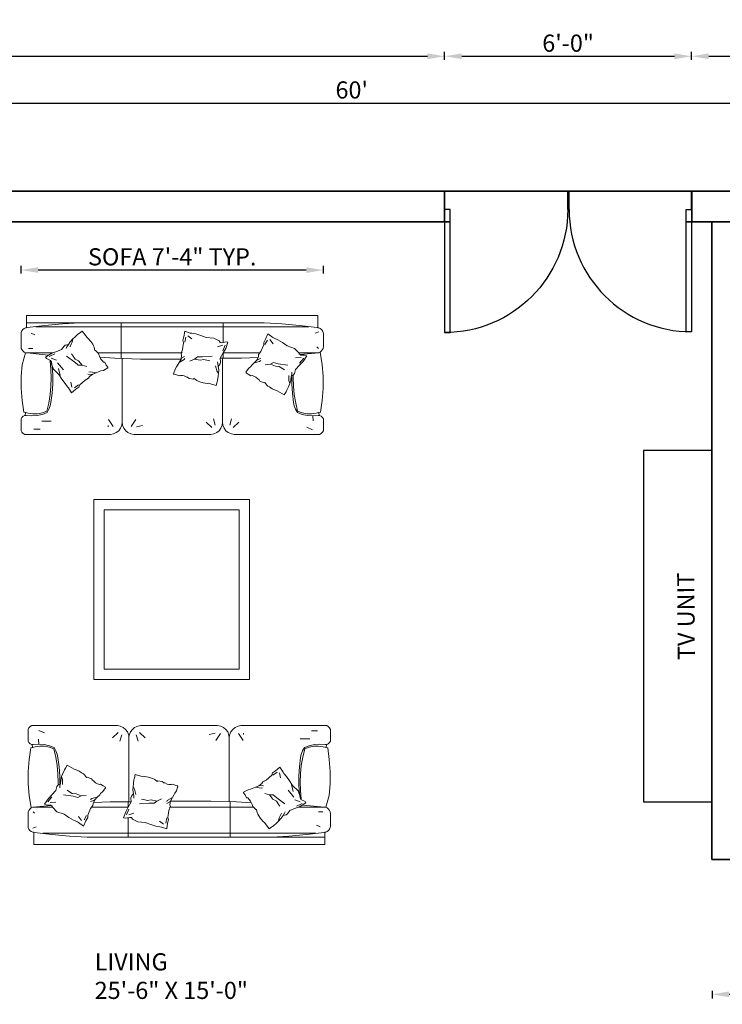
# Model space of a CAD drawing. Units: inches. Extents: x -48 to 817, y -530 to 78.
# Tile 6 of 7: x 266 to 470, y -225 to 62. Entities that reach past the tile are written whole.
import ezdxf

# ---------------------------------------------------------------- set-up
doc = ezdxf.new("R2010")
doc.units = ezdxf.units.IN
for name, color, linetype, lineweight in [('A-ANNO-DIMS', 2, 'Continuous', 18), ('A-AREA-IDEN', 7, 'Continuous', 18), ('A-DOOR', 3, 'Continuous', 25), ('A-FLOR-CASE', 8, 'Continuous', 25), ('A-WALL', 7, 'Continuous', 35), ('furn', 8, 'Continuous', 18), ('txt', 7, 'Continuous', 18)]:
    doc.layers.add(name, color=color, linetype=linetype, lineweight=lineweight)
doc.styles.get("Standard").update_dxf_attribs({"font": 'arial.ttf'})
doc.dimstyles.new('ISO-25', dxfattribs={"dimtxt": 5, "dimasz": 5, "dimexe": 1.25, "dimexo": 0.625, "dimtad": 1, "dimlunit": 3, "dimtxsty": 'Standard', "dimcen": 2.5, "dimadec": 0, "dimazin": 0, "dimtfac": 1, "dimtmove": 0, "dimatfit": 3, "dimfxl": 1, "dimfxlon": 1, "dimarcsym": 0})

# ---------------------------------------------------------------- blocks, each defined once
blk = doc.blocks.new('*U2')
for p, q in [((0, 0), (0, -6)), ((40, 0), (40, -6))]:
    blk.add_line(p, q)
blk.add_lwpolyline([(0, 0), (0, 40), (1.75, 40), (1.75, 0)], close=True)
blk.add_arc((0, 0), 40, 0, 90)
blk = doc.blocks.new('sofa-43')
at = {"color": 0, "linetype": 'ByBlock'}
for p, q in [((-0.015, 0.947), (-0.028, 0.939)), ((-0.028, 0.939), (-0.015, 0.947)), ((-0.003, 0.947), (-0.015, 0.947)), ((-0.015, 0.947), (-0.003, 0.947)), ((0.665, 0.947), (-0.003, 0.947)), ((-0.003, 0.947), (0.665, 0.947)), ((0.687, 0.942), (0.665, 0.947)), ((0.687, 0.942), (0.665, 0.947)), ((0.712, 0.932), (0.687, 0.942)), ((0.712, 0.932), (0.687, 0.942)), ((0.827, 0.942), (0.802, 0.932)), ((0.802, 0.932), (0.827, 0.942)), ((0.85, 0.947), (0.827, 0.942)), ((0.827, 0.942), (0.85, 0.947)), ((1.462, 0.947), (0.85, 0.947)), ((0.85, 0.947), (1.462, 0.947)), ((1.487, 0.942), (1.462, 0.947)), ((1.487, 0.942), (1.462, 0.947)), ((1.509, 0.932), (1.487, 0.942)), ((1.509, 0.932), (1.487, 0.942)), ((1.624, 0.942), (1.602, 0.932)), ((1.602, 0.932), (1.624, 0.942)), ((1.647, 0.947), (1.624, 0.942)), ((1.624, 0.942), (1.647, 0.947)), ((2.317, 0.947), (1.647, 0.947)), ((1.647, 0.947), (2.317, 0.947)), ((2.329, 0.947), (2.317, 0.947)), ((2.329, 0.947), (2.317, 0.947)), ((2.342, 0.939), (2.329, 0.947)), ((2.342, 0.939), (2.329, 0.947)), ((-0.038, 0.929), (-0.045, 0.917)), ((-0.045, 0.917), (-0.038, 0.929)), ((-0.045, 0.917), (-0.045, 0.824)), ((-0.045, 0.917), (-0.045, 0.824)), ((-0.028, 0.939), (-0.038, 0.929)), ((-0.038, 0.929), (-0.028, 0.939)), ((0.042, 0.909), (0.087, 0.889)), ((0.672, 0.892), (0.627, 0.849)), ((0.7, 0.874), (0.685, 0.824)), ((0.73, 0.917), (0.712, 0.932)), ((0.73, 0.917), (0.712, 0.932)), ((0.745, 0.897), (0.73, 0.917)), ((0.745, 0.897), (0.73, 0.917)), ((0.755, 0.872), (0.745, 0.897)), ((0.755, 0.872), (0.745, 0.897)), ((0.757, 0.849), (0.755, 0.872)), ((0.757, 0.849), (0.755, 0.872)), ((0.76, 0.872), (0.757, 0.849)), ((0.757, 0.849), (0.76, 0.872)), ((0.77, 0.897), (0.76, 0.872)), ((0.76, 0.872), (0.77, 0.897)), ((0.785, 0.917), (0.77, 0.897)), ((0.77, 0.897), (0.785, 0.917)), ((0.802, 0.932), (0.785, 0.917)), ((0.785, 0.917), (0.802, 0.932)), ((0.815, 0.874), (0.83, 0.824)), ((0.842, 0.892), (0.887, 0.849)), ((1.442, 0.887), (1.394, 0.877)), ((1.484, 0.884), (1.447, 0.829)), ((1.527, 0.917), (1.509, 0.932)), ((1.527, 0.917), (1.509, 0.932)), ((1.542, 0.897), (1.527, 0.917)), ((1.542, 0.897), (1.527, 0.917)), ((1.552, 0.872), (1.542, 0.897)), ((1.552, 0.872), (1.542, 0.897)), ((1.554, 0.849), (1.552, 0.872)), ((1.554, 0.849), (1.552, 0.872)), ((1.557, 0.872), (1.554, 0.849)), ((1.554, 0.849), (1.557, 0.872)), ((1.567, 0.897), (1.557, 0.872)), ((1.557, 0.872), (1.567, 0.897)), ((1.582, 0.917), (1.567, 0.897)), ((1.567, 0.897), (1.582, 0.917)), ((1.602, 0.932), (1.582, 0.917)), ((1.582, 0.917), (1.602, 0.932)), ((1.627, 0.884), (1.664, 0.829)), ((1.667, 0.887), (1.667, 0.877)), ((2.257, 0.904), (2.207, 0.904)), ((2.352, 0.929), (2.342, 0.939)), ((2.352, 0.929), (2.342, 0.939)), ((2.359, 0.917), (2.352, 0.929)), ((2.359, 0.917), (2.352, 0.929)), ((2.359, 0.824), (2.359, 0.917)), ((2.359, 0.917), (2.359, 0.824)), ((-0.045, 0.824), (-0.038, 0.812)), ((-0.045, 0.824), (-0.038, 0.812)), ((-0.038, 0.812), (-0.028, 0.802)), ((-0.038, 0.812), (-0.028, 0.802)), ((-0.028, 0.802), (-0.015, 0.797)), ((-0.028, 0.802), (-0.015, 0.797)), ((-0.015, 0.797), (-0.0064, 0.7737)), ((-0.015, 0.797), (-0.003, 0.797)), ((-0.0064, 0.7737), (-0.015, 0.797)), ((0.04, 0.799), (-0.003, 0.797)), ((0.04, 0.799), (0.037, 0.839)), ((0.082, 0.797), (0.04, 0.799)), ((0.125, 0.787), (0.082, 0.797)), ((0.162, 0.772), (0.125, 0.787)), ((0.757, 0.345), (0.757, 0.849)), ((1.554, 0.345), (1.554, 0.849)), ((2.194, 0.842), (2.119, 0.842)), ((2.152, 0.772), (2.189, 0.787)), ((2.189, 0.787), (2.232, 0.797)), ((2.232, 0.797), (2.274, 0.799)), ((2.274, 0.799), (2.317, 0.797)), ((2.329, 0.797), (2.317, 0.797)), ((2.3218, 0.7734), (2.329, 0.797)), ((2.3218, 0.7734), (2.329, 0.797)), ((2.329, 0.797), (2.342, 0.802)), ((2.342, 0.802), (2.329, 0.797)), ((2.342, 0.802), (2.352, 0.812)), ((2.352, 0.812), (2.342, 0.802)), ((2.352, 0.812), (2.359, 0.824)), ((2.359, 0.824), (2.352, 0.812)), ((-0.023, 0.769), (-0.035, 0.677)), ((-0.023, 0.769), (-0.035, 0.677)), ((0.012, 0.779), (-0.023, 0.769)), ((-0.0064, 0.7737), (-0.023, 0.769)), ((0.05, 0.782), (0.012, 0.779)), ((0.087, 0.782), (0.05, 0.782)), ((0.125, 0.774), (0.087, 0.782)), ((0.16, 0.762), (0.125, 0.774)), ((0.175, 0.697), (0.16, 0.762)), ((0.177, 0.747), (0.162, 0.772)), ((0.187, 0.719), (0.177, 0.747)), ((0.192, 0.692), (0.187, 0.719)), ((2.122, 0.692), (2.127, 0.719)), ((2.127, 0.719), (2.137, 0.747)), ((2.137, 0.747), (2.152, 0.772)), ((2.139, 0.697), (2.154, 0.762)), ((2.154, 0.762), (2.189, 0.774)), ((2.189, 0.774), (2.227, 0.782)), ((2.227, 0.782), (2.264, 0.782)), ((2.264, 0.782), (2.302, 0.779)), ((2.302, 0.779), (2.337, 0.769)), ((2.337, 0.769), (2.3218, 0.7734)), ((2.349, 0.677), (2.337, 0.769)), ((2.337, 0.769), (2.349, 0.677)), ((-0.035, 0.677), (-0.043, 0.582)), ((-0.035, 0.677), (-0.043, 0.582)), ((0.187, 0.629), (0.175, 0.697)), ((0.192, 0.562), (0.187, 0.629)), ((0.202, 0.619), (0.192, 0.692)), ((0.267, 0.632), (0.252, 0.607)), ((0.322, 0.599), (0.267, 0.632)), ((2.112, 0.619), (2.122, 0.692)), ((2.122, 0.562), (2.127, 0.629)), ((2.127, 0.629), (2.139, 0.697)), ((2.357, 0.582), (2.349, 0.677)), ((2.349, 0.677), (2.357, 0.582)), ((-0.043, 0.582), (-0.043, 0.484)), ((-0.043, 0.582), (-0.043, 0.484)), ((0.195, 0.497), (0.192, 0.562)), ((0.207, 0.547), (0.202, 0.619)), ((0.232, 0.567), (0.222, 0.542)), ((0.245, 0.594), (0.232, 0.567)), ((0.252, 0.607), (0.245, 0.594)), ((0.332, 0.597), (0.322, 0.599)), ((0.362, 0.584), (0.332, 0.597)), ((0.385, 0.569), (0.362, 0.584)), ((0.397, 0.562), (0.385, 0.569)), ((0.405, 0.554), (0.397, 0.562)), ((0.42, 0.534), (0.405, 0.554)), ((0.807, 0.557), (0.8, 0.529)), ((0.87, 0.539), (0.807, 0.557)), ((1.892, 0.552), (1.849, 0.514)), ((1.899, 0.572), (1.892, 0.552)), ((1.922, 0.587), (1.899, 0.572)), ((1.934, 0.577), (1.902, 0.552)), ((1.957, 0.617), (1.922, 0.587)), ((1.954, 0.572), (1.962, 0.532)), ((1.982, 0.577), (1.957, 0.617)), ((1.989, 0.567), (1.982, 0.577)), ((2.009, 0.542), (1.989, 0.567)), ((2.107, 0.547), (2.112, 0.619)), ((2.119, 0.497), (2.122, 0.562)), ((2.357, 0.484), (2.357, 0.582)), ((2.357, 0.582), (2.357, 0.484)), ((-0.043, 0.484), (-0.035, 0.392)), ((-0.043, 0.484), (-0.035, 0.392)), ((0.192, 0.472), (0.185, 0.462)), ((0.212, 0.487), (0.192, 0.472)), ((0.195, 0.482), (0.195, 0.497)), ((0.207, 0.492), (0.207, 0.547)), ((0.207, 0.467), (0.212, 0.487)), ((0.215, 0.514), (0.212, 0.487)), ((0.222, 0.542), (0.215, 0.514)), ((0.222, 0.542), (0.23, 0.519)), ((0.23, 0.519), (0.23, 0.497)), ((0.23, 0.497), (0.23, 0.477)), ((0.425, 0.537), (0.42, 0.534)), ((0.46, 0.524), (0.425, 0.537)), ((0.467, 0.512), (0.46, 0.524)), ((0.475, 0.507), (0.467, 0.512)), ((0.492, 0.492), (0.475, 0.507)), ((0.507, 0.484), (0.492, 0.492)), ((0.522, 0.479), (0.507, 0.484)), ((0.532, 0.482), (0.522, 0.479)), ((0.552, 0.467), (0.532, 0.482)), ((0.792, 0.484), (0.79, 0.462)), ((0.797, 0.517), (0.792, 0.484)), ((0.8, 0.529), (0.797, 0.517)), ((0.88, 0.542), (0.87, 0.539)), ((0.912, 0.537), (0.88, 0.542)), ((0.937, 0.529), (0.912, 0.537)), ((0.952, 0.524), (0.937, 0.529)), ((0.962, 0.519), (0.952, 0.524)), ((0.982, 0.502), (0.962, 0.519)), ((0.987, 0.507), (0.982, 0.502)), ((1.022, 0.502), (0.987, 0.507)), ((1.035, 0.492), (1.022, 0.502)), ((1.042, 0.492), (1.035, 0.492)), ((1.062, 0.482), (1.042, 0.492)), ((1.074, 0.477), (1.062, 0.482)), ((1.092, 0.477), (1.074, 0.477)), ((1.102, 0.482), (1.092, 0.477)), ((1.124, 0.472), (1.102, 0.482)), ((1.144, 0.467), (1.124, 0.472)), ((1.814, 0.487), (1.789, 0.467)), ((1.789, 0.467), (1.802, 0.47)), ((1.802, 0.47), (1.827, 0.467)), ((1.822, 0.499), (1.814, 0.487)), ((1.849, 0.514), (1.822, 0.499)), ((1.827, 0.504), (1.832, 0.502)), ((2.034, 0.507), (2.009, 0.542)), ((2.057, 0.47), (2.034, 0.507)), ((2.062, 0.422), (2.049, 0.479)), ((2.102, 0.427), (2.057, 0.47)), ((2.107, 0.474), (2.107, 0.547)), ((2.112, 0.405), (2.107, 0.474)), ((2.122, 0.43), (2.119, 0.497)), ((2.349, 0.392), (2.357, 0.484)), ((2.357, 0.484), (2.349, 0.392)), ((-0.035, 0.392), (-0.02, 0.292)), ((-0.035, 0.392), (-0.02, 0.292)), ((0.145, 0.395), (0.117, 0.367)), ((0.177, 0.43), (0.145, 0.395)), ((0.185, 0.462), (0.177, 0.43)), ((0.207, 0.452), (0.207, 0.467)), ((0.237, 0.397), (0.315, 0.385)), ((0.277, 0.425), (0.265, 0.432)), ((0.307, 0.407), (0.277, 0.425)), ((0.337, 0.405), (0.307, 0.407)), ((0.377, 0.387), (0.337, 0.405)), ((0.377, 0.387), (0.417, 0.392)), ((0.505, 0.377), (0.525, 0.397)), ((0.525, 0.397), (0.532, 0.407)), ((0.532, 0.407), (0.55, 0.422)), ((0.55, 0.422), (0.572, 0.452)), ((0.57, 0.457), (0.552, 0.467)), ((0.572, 0.452), (0.57, 0.457)), ((0.792, 0.407), (0.777, 0.385)), ((0.79, 0.462), (0.787, 0.432)), ((0.787, 0.432), (0.792, 0.407)), ((0.79, 0.462), (0.802, 0.442)), ((0.795, 0.382), (0.792, 0.407)), ((0.802, 0.442), (0.807, 0.42)), ((0.807, 0.42), (0.812, 0.4)), ((1.102, 0.375), (1.117, 0.4)), ((1.117, 0.4), (1.122, 0.41)), ((1.122, 0.41), (1.134, 0.427)), ((1.134, 0.427), (1.147, 0.465)), ((1.147, 0.465), (1.144, 0.467)), ((1.704, 0.437), (1.669, 0.417)), ((1.669, 0.417), (1.669, 0.412)), ((1.669, 0.412), (1.682, 0.395)), ((1.682, 0.395), (1.692, 0.372)), ((1.724, 0.442), (1.704, 0.437)), ((1.737, 0.447), (1.724, 0.442)), ((1.762, 0.457), (1.737, 0.447)), ((1.789, 0.467), (1.762, 0.457)), ((1.762, 0.457), (1.807, 0.45)), ((1.807, 0.45), (1.819, 0.452)), ((1.874, 0.397), (1.837, 0.407)), ((1.874, 0.397), (1.902, 0.362)), ((1.904, 0.397), (1.874, 0.397)), ((1.932, 0.372), (1.904, 0.397)), ((2.069, 0.377), (2.022, 0.432)), ((2.119, 0.382), (2.102, 0.427)), ((2.117, 0.375), (2.112, 0.405)), ((2.127, 0.362), (2.122, 0.43)), ((2.322, 0.297), (2.349, 0.392)), ((2.349, 0.392), (2.322, 0.297)), ((0.117, 0.367), (0.087, 0.322)), ((0.087, 0.322), (0.1, 0.317)), ((0.1, 0.317), (0.135, 0.315)), ((0.112, 0.34), (0.145, 0.38)), ((0.132, 0.335), (0.177, 0.337)), ((0.135, 0.315), (0.147, 0.307)), ((0.315, 0.385), (0.352, 0.375)), ((0.352, 0.375), (0.377, 0.387)), ((0.462, 0.367), (0.452, 0.36)), ((0.477, 0.35), (0.452, 0.342)), ((0.505, 0.377), (0.462, 0.367)), ((0.47, 0.312), (0.472, 0.327)), ((0.472, 0.327), (0.485, 0.357)), ((0.607, 0.34), (0.475, 0.335)), ((0.485, 0.357), (0.477, 0.35)), ((0.485, 0.357), (0.505, 0.377)), ((0.775, 0.34), (0.607, 0.34)), ((0.775, 0.34), (0.752, 0.297)), ((0.752, 0.297), (0.752, 0.34)), ((0.777, 0.385), (0.772, 0.372)), ((0.772, 0.372), (0.775, 0.34)), ((0.797, 0.37), (0.795, 0.382)), ((0.84, 0.325), (0.917, 0.33)), ((0.872, 0.36), (0.857, 0.362)), ((0.905, 0.35), (0.872, 0.36)), ((0.935, 0.357), (0.905, 0.35)), ((0.917, 0.33), (0.957, 0.33)), ((0.98, 0.347), (0.935, 0.357)), ((0.957, 0.33), (0.98, 0.347)), ((0.98, 0.347), (1.017, 0.365)), ((1.062, 0.352), (1.057, 0.342)), ((1.082, 0.34), (1.059, 0.327)), ((1.102, 0.375), (1.062, 0.352)), ((1.087, 0.347), (1.082, 0.34)), ((1.082, 0.317), (1.087, 0.347)), ((1.087, 0.302), (1.082, 0.317)), ((1.087, 0.347), (1.102, 0.375)), ((1.409, 0.347), (1.087, 0.347)), ((1.612, 0.34), (1.409, 0.347)), ((1.562, 0.06), (1.562, 0.34)), ((1.732, 0.332), (1.612, 0.34)), ((1.692, 0.372), (1.702, 0.372)), ((1.702, 0.372), (1.714, 0.36)), ((1.714, 0.36), (1.724, 0.347)), ((1.724, 0.347), (1.734, 0.325)), ((1.734, 0.325), (1.737, 0.32)), ((1.737, 0.32), (1.742, 0.302)), ((1.902, 0.362), (1.929, 0.347)), ((1.929, 0.347), (1.949, 0.317)), ((1.997, 0.325), (1.932, 0.372)), ((1.949, 0.317), (1.957, 0.307)), ((2.119, 0.34), (2.077, 0.357)), ((2.134, 0.327), (2.089, 0.305)), ((2.117, 0.317), (2.114, 0.317)), ((2.117, 0.37), (2.119, 0.382)), ((2.124, 0.36), (2.117, 0.37)), ((2.119, 0.302), (2.164, 0.332)), ((2.157, 0.342), (2.124, 0.36)), ((2.129, 0.357), (2.127, 0.362)), ((2.144, 0.315), (2.137, 0.317)), ((2.137, 0.315), (2.137, 0.317)), ((2.309, 0.297), (2.144, 0.315)), ((2.164, 0.332), (2.157, 0.342)), ((-0.043, 0.262), (-0.045, 0.247)), ((-0.043, 0.262), (-0.045, 0.247)), ((-0.045, 0.247), (-0.045, 0.147)), ((-0.045, 0.247), (-0.045, 0.147)), ((-0.038, 0.272), (-0.043, 0.262)), ((-0.038, 0.272), (-0.043, 0.262)), ((-0.03, 0.282), (-0.038, 0.272)), ((-0.03, 0.282), (-0.038, 0.272)), ((-0.02, 0.292), (-0.03, 0.282)), ((-0.02, 0.292), (-0.03, 0.282)), ((-0.008, 0.297), (-0.02, 0.292)), ((0.14, 0.312), (-0.008, 0.297)), ((-0.008, 0.297), (0.15, 0.297)), ((0.005, 0.297), (-0.008, 0.297)), ((-0.005, 0.262), (0.007, 0.25)), ((0.147, 0.307), (0.152, 0.295)), ((0.152, 0.295), (0.185, 0.262)), ((0.185, 0.262), (0.242, 0.242)), ((0.242, 0.242), (0.28, 0.215)), ((0.43, 0.235), (0.452, 0.287)), ((0.43, 0.215), (0.43, 0.235)), ((0.452, 0.287), (0.47, 0.312)), ((0.46, 0.297), (0.752, 0.297)), ((0.467, 0.307), (0.462, 0.307)), ((0.732, 0.262), (0.715, 0.212)), ((0.752, 0.297), (0.732, 0.262)), ((0.737, 0.237), (0.755, 0.282)), ((0.755, 0.237), (0.797, 0.25)), ((1.067, 0.217), (1.074, 0.272)), ((1.074, 0.272), (1.087, 0.302)), ((1.084, 0.297), (1.079, 0.292)), ((1.0855, 0.2985), (1.084, 0.297)), ((1.084, 0.297), (1.0848, 0.297)), ((1.084, 0.297), (1.562, 0.297)), ((1.0848, 0.297), (1.0855, 0.2985)), ((1.562, 0.297), (1.747, 0.297)), ((1.742, 0.302), (1.767, 0.28)), ((1.767, 0.28), (1.772, 0.28)), ((1.772, 0.28), (1.777, 0.252)), ((1.777, 0.252), (1.782, 0.242)), ((1.782, 0.242), (1.789, 0.23)), ((1.959, 0.23), (1.969, 0.25)), ((1.994, 0.25), (1.982, 0.232)), ((1.982, 0.232), (2.007, 0.237)), ((1.999, 0.262), (1.994, 0.25)), ((2.007, 0.237), (2.017, 0.245)), ((2.017, 0.245), (2.037, 0.272)), ((2.037, 0.272), (2.082, 0.29)), ((2.082, 0.29), (2.119, 0.302)), ((2.104, 0.297), (2.309, 0.297)), ((2.299, 0.262), (2.264, 0.262)), ((2.322, 0.297), (2.309, 0.297)), ((2.334, 0.292), (2.322, 0.297)), ((2.334, 0.292), (2.322, 0.297)), ((2.344, 0.282), (2.334, 0.292)), ((2.344, 0.282), (2.334, 0.292)), ((2.352, 0.272), (2.344, 0.282)), ((2.352, 0.272), (2.344, 0.282)), ((2.357, 0.262), (2.352, 0.272)), ((2.357, 0.262), (2.352, 0.272)), ((2.359, 0.247), (2.357, 0.262)), ((2.359, 0.247), (2.357, 0.262)), ((2.359, 0.147), (2.359, 0.247)), ((2.359, 0.147), (2.359, 0.247)), ((0.28, 0.215), (0.317, 0.195)), ((0.317, 0.195), (0.347, 0.182)), ((0.347, 0.182), (0.357, 0.175)), ((0.38, 0.192), (0.355, 0.225)), ((0.357, 0.175), (0.397, 0.147)), ((0.397, 0.147), (0.415, 0.19)), ((0.4, 0.197), (0.42, 0.232)), ((0.415, 0.19), (0.43, 0.215)), ((0.715, 0.212), (0.727, 0.21)), ((0.727, 0.21), (0.765, 0.217)), ((0.752, 0.06), (0.752, 0.215)), ((0.765, 0.217), (0.777, 0.215)), ((0.777, 0.215), (0.785, 0.202)), ((0.785, 0.202), (0.827, 0.18)), ((0.827, 0.18), (0.887, 0.175)), ((0.887, 0.175), (0.93, 0.16)), ((0.93, 0.16), (0.97, 0.147)), ((1.032, 0.162), (1, 0.187)), ((1.05, 0.172), (1.057, 0.212)), ((1.057, 0.125), (1.064, 0.17)), ((1.064, 0.17), (1.072, 0.197)), ((1.072, 0.197), (1.067, 0.217)), ((1.789, 0.23), (1.804, 0.207)), ((1.804, 0.207), (1.827, 0.182)), ((1.827, 0.182), (1.834, 0.177)), ((1.834, 0.177), (1.872, 0.125)), ((1.907, 0.15), (1.929, 0.17)), ((1.929, 0.17), (1.947, 0.187)), ((1.947, 0.187), (1.952, 0.212)), ((1.947, 0.187), (1.967, 0.21)), ((1.952, 0.212), (1.959, 0.23)), ((1.967, 0.21), (1.982, 0.232)), ((-0.045, 0.147), (-0.043, 0.135)), ((-0.045, 0.147), (-0.043, 0.135)), ((-0.043, 0.135), (-0.038, 0.122)), ((-0.043, 0.135), (-0.038, 0.122)), ((-0.038, 0.122), (-0.03, 0.112)), ((-0.038, 0.122), (-0.03, 0.112)), ((-0.03, 0.112), (-0.02, 0.105)), ((-0.03, 0.112), (-0.02, 0.105)), ((-0.02, 0.105), (-0.008, 0.1)), ((-0.02, 0.105), (-0.008, 0.1)), ((-0.008, 0.132), (0.02, 0.142)), ((-0.008, 0.1), (0, 0.0982)), ((-0.008, 0.1), (0.005, 0.097)), ((0, 0.1), (0, 0)), ((0, 0.0982), (0, 0)), ((0.005, 0.097), (0.145, 0.08)), ((0.072, 0.09), (0.752, 0.09)), ((0.145, 0.08), (0.285, 0.067)), ((0.752, 0.09), (1.562, 0.09)), ((0.97, 0.147), (1.002, 0.142)), ((1.002, 0.142), (1.015, 0.14)), ((1.015, 0.14), (1.057, 0.125)), ((1.562, 0.09), (2.242, 0.09)), ((1.872, 0.125), (1.894, 0.142)), ((1.894, 0.142), (1.907, 0.15)), ((2.029, 0.067), (2.169, 0.08)), ((2.169, 0.08), (2.309, 0.097)), ((2.277, 0.142), (2.249, 0.155)), ((2.309, 0.097), (2.322, 0.1)), ((2.314, 0.0982), (2.322, 0.1)), ((2.314, 0.1), (2.314, 0)), ((2.314, 0), (2.314, 0.0982)), ((2.322, 0.1), (2.334, 0.105)), ((2.322, 0.1), (2.334, 0.105)), ((2.334, 0.105), (2.344, 0.112)), ((2.334, 0.105), (2.344, 0.112)), ((2.344, 0.112), (2.352, 0.122)), ((2.344, 0.112), (2.352, 0.122)), ((2.352, 0.122), (2.357, 0.135)), ((2.352, 0.122), (2.357, 0.135)), ((2.357, 0.135), (2.359, 0.147)), ((2.357, 0.135), (2.359, 0.147)), ((0, 0), (2.314, 0)), ((0, 0), (2.314, 0)), ((0.285, 0.067), (0.425, 0.06)), ((0.425, 0.06), (2.314, 0.06)), ((1.889, 0.06), (2.029, 0.067))]:
    blk.add_line(p, q, dxfattribs=at)
blk = doc.blocks.new('*D9')
at = {"layer": 'A-ANNO-DIMS', "color": 0, "lineweight": -2, "transparency": 16777216}
for p, q in [((2.43, 36.38), (2.43, 38.63)), ((7.43, 37.38), (717.43, 37.38)), ((722.43, 36.38), (722.43, 38.63))]:
    blk.add_line(p, q, dxfattribs=at)
at = {"layer": 'A-ANNO-DIMS', "color": 0, "transparency": 16777216}
for points in [[(7.43, 38.21), (7.43, 36.54), (2.43, 37.38)], [(717.43, 38.21), (717.43, 36.54), (722.43, 37.38)]]:
    blk.add_solid(points, dxfattribs=at)
at = {"layer": 'Defpoints', "color": 0, "transparency": 16777216}
for p in [(722.43, 37.38), (2.43, 11.72), (722.43, 11.72)]:
    blk.add_point(p, dxfattribs=at)
at = {"layer": 'A-ANNO-DIMS', "color": 0, "transparency": 16777216, "insert": (362.43, 40.55), "char_height": 5, "attachment_point": 5}
blk.add_mtext("60'", dxfattribs=at)
blk = doc.blocks.new('*D26')
at = {"layer": 'A-ANNO-DIMS', "color": 0, "lineweight": -2, "transparency": 16777216}
for p, q in [((266.04, -12.33), (266.04, -10.08)), ((349.18, -11.33), (271.04, -11.33)), ((354.18, -12.33), (354.18, -10.08))]:
    blk.add_line(p, q, dxfattribs=at)
at = {"layer": 'A-ANNO-DIMS', "color": 0, "transparency": 16777216}
for points in [[(271.04, -10.5), (271.04, -12.17), (266.04, -11.33)], [(349.18, -10.5), (349.18, -12.17), (354.18, -11.33)]]:
    blk.add_solid(points, dxfattribs=at)
at = {"layer": 'Defpoints', "color": 0, "transparency": 16777216}
for p in [(266.04, -11.33), (266.04, -24.56), (354.18, -24.56)]:
    blk.add_point(p, dxfattribs=at)
at = {"layer": 'A-ANNO-DIMS', "color": 0, "transparency": 16777216, "insert": (310.11, -8.12), "char_height": 5, "attachment_point": 5}
blk.add_mtext('SOFA 7\'-4" TYP.', dxfattribs=at)
blk = doc.blocks.new('*D27')
at = {"layer": 'A-ANNO-DIMS', "color": 0, "lineweight": -2, "transparency": 16777216}
for p, q in [((253.82, -24.56), (251.57, -24.56)), ((252.82, -29.56), (252.82, -54.28)), ((253.82, -59.28), (251.57, -59.28)), ((252.82, -59.28), (252.82, -111.62))]:
    blk.add_line(p, q, dxfattribs=at)
at = {"layer": 'A-ANNO-DIMS', "color": 0, "transparency": 16777216}
for points in [[(251.99, -29.56), (253.65, -29.56), (252.82, -24.56)], [(251.99, -54.28), (253.65, -54.28), (252.82, -59.28)]]:
    blk.add_solid(points, dxfattribs=at)
at = {"layer": 'Defpoints', "color": 0, "transparency": 16777216}
for p in [(266.04, -24.56), (252.82, -59.28), (266.04, -59.28)]:
    blk.add_point(p, dxfattribs=at)
at = {"layer": 'A-ANNO-DIMS', "color": 0, "transparency": 16777216, "insert": (249.61, -87.95), "char_height": 5, "attachment_point": 5, "rotation": 90}
blk.add_mtext('2\'-10 1/2" TYP.', dxfattribs=at)
blk = doc.blocks.new('*D44')
at = {"layer": 'A-ANNO-DIMS', "color": 0, "lineweight": -2, "transparency": 16777216}
for p, q in [((389.5, 50.02), (389.5, 52.27)), ((461.47, 50.02), (461.47, 52.27)), ((394.5, 51.02), (456.47, 51.02))]:
    blk.add_line(p, q, dxfattribs=at)
at = {"layer": 'A-ANNO-DIMS', "color": 0, "transparency": 16777216}
for points in [[(394.5, 51.86), (394.5, 50.19), (389.5, 51.02)], [(456.47, 51.86), (456.47, 50.19), (461.47, 51.02)]]:
    blk.add_solid(points, dxfattribs=at)
at = {"layer": 'Defpoints', "color": 0, "transparency": 16777216}
for p in [(461.47, 51.02), (389.5, 11.72), (461.47, 11.72)]:
    blk.add_point(p, dxfattribs=at)
at = {"layer": 'A-ANNO-DIMS', "color": 0, "transparency": 16777216, "insert": (425.49, 54.2), "char_height": 5, "attachment_point": 5}
blk.add_mtext('6\'-0"', dxfattribs=at)
blk = doc.blocks.new('*D48')
at = {"layer": 'A-ANNO-DIMS', "color": 0, "lineweight": -2, "transparency": 16777216}
for p, q in [((105.2, 50.02), (105.2, 52.27)), ((389.5, 50.02), (389.5, 52.27)), ((110.2, 51.02), (384.5, 51.02))]:
    blk.add_line(p, q, dxfattribs=at)
at = {"layer": 'A-ANNO-DIMS', "color": 0, "transparency": 16777216}
for points in [[(110.2, 51.86), (110.2, 50.19), (105.2, 51.02)], [(384.5, 51.86), (384.5, 50.19), (389.5, 51.02)]]:
    blk.add_solid(points, dxfattribs=at)
at = {"layer": 'Defpoints', "color": 0, "transparency": 16777216}
for p in [(389.5, 51.02), (105.2, 11.72), (389.5, 11.72)]:
    blk.add_point(p, dxfattribs=at)
at = {"layer": 'A-ANNO-DIMS', "color": 0, "transparency": 16777216, "insert": (247.35, 54.24), "char_height": 5, "attachment_point": 5}
blk.add_mtext('23\'-8 1/2"', dxfattribs=at)
blk = doc.blocks.new('*D49')
at = {"layer": 'A-ANNO-DIMS', "color": 0, "lineweight": -2, "transparency": 16777216}
for p, q in [((461.47, 50.02), (461.47, 52.27)), ((509.58, 50.02), (509.58, 52.27)), ((466.47, 51.02), (504.58, 51.02))]:
    blk.add_line(p, q, dxfattribs=at)
at = {"layer": 'A-ANNO-DIMS', "color": 0, "transparency": 16777216}
for points in [[(466.47, 51.86), (466.47, 50.19), (461.47, 51.02)], [(504.58, 51.86), (504.58, 50.19), (509.58, 51.02)]]:
    blk.add_solid(points, dxfattribs=at)
at = {"layer": 'Defpoints', "color": 0, "transparency": 16777216}
for p in [(509.58, 51.02), (461.47, 11.72), (509.58, 11.72)]:
    blk.add_point(p, dxfattribs=at)
at = {"layer": 'A-ANNO-DIMS', "color": 0, "transparency": 16777216, "insert": (485.53, 54.2), "char_height": 5, "attachment_point": 5}
blk.add_mtext('4\'-0"', dxfattribs=at)
blk = doc.blocks.new('*D58')
at = {"layer": 'A-ANNO-DIMS', "color": 0, "lineweight": -2, "transparency": 16777216}
for p, q in [((811.62, -33.28), (813.87, -33.28)), ((812.62, -38.28), (812.62, -100.61)), ((811.62, -105.61), (813.87, -105.61))]:
    blk.add_line(p, q, dxfattribs=at)
at = {"layer": 'A-ANNO-DIMS', "color": 0, "transparency": 16777216}
for points in [[(811.79, -38.28), (813.45, -38.28), (812.62, -33.28)], [(811.79, -100.61), (813.45, -100.61), (812.62, -105.61)]]:
    blk.add_solid(points, dxfattribs=at)
at = {"layer": 'Defpoints', "color": 0, "transparency": 16777216}
for p in [(161.43, -33.28), (161.43, -105.61), (812.62, -105.61)]:
    blk.add_point(p, dxfattribs=at)
at = {"layer": 'A-ANNO-DIMS', "color": 0, "transparency": 16777216, "insert": (809.41, -69.44), "char_height": 5, "attachment_point": 5, "rotation": 90}
blk.add_mtext('6\'-0 1/2"', dxfattribs=at)
blk = doc.blocks.new('*D60')
at = {"layer": 'A-ANNO-DIMS', "color": 0, "lineweight": -2, "transparency": 16777216}
for p, q in [((467.43, -221.58), (467.43, -223.83)), ((511.25, -222.58), (472.43, -222.58)), ((516.25, -221.58), (516.25, -223.83))]:
    blk.add_line(p, q, dxfattribs=at)
at = {"layer": 'A-ANNO-DIMS', "color": 0, "transparency": 16777216}
for points in [[(472.43, -221.74), (472.43, -223.41), (467.43, -222.58)], [(511.25, -221.74), (511.25, -223.41), (516.25, -222.58)]]:
    blk.add_solid(points, dxfattribs=at)
at = {"layer": 'Defpoints', "color": 0, "transparency": 16777216}
for p in [(467.43, -183.28), (516.25, -183.28), (467.43, -222.58)]:
    blk.add_point(p, dxfattribs=at)
at = {"layer": 'A-ANNO-DIMS', "color": 0, "transparency": 16777216, "insert": (491.84, -219.44), "char_height": 5, "attachment_point": 5}
blk.add_mtext('4\'-1"', dxfattribs=at)
blk = doc.blocks.new('*D68')
at = {"layer": 'A-ANNO-DIMS', "color": 0, "lineweight": -2, "transparency": 16777216}
for p, q in [((-35.87, -153.28), (-38.12, -153.28)), ((-36.87, -158.28), (-36.87, -172.28)), ((-35.87, -177.28), (-38.12, -177.28))]:
    blk.add_line(p, q, dxfattribs=at)
at = {"layer": 'A-ANNO-DIMS', "color": 0, "transparency": 16777216}
for points in [[(-37.71, -158.28), (-36.04, -158.28), (-36.87, -153.28)], [(-37.71, -172.28), (-36.04, -172.28), (-36.87, -177.28)]]:
    blk.add_solid(points, dxfattribs=at)
at = {"layer": 'Defpoints', "color": 0, "transparency": 16777216}
for p in [(570.33, -153.28), (-36.87, -177.28), (570.33, -177.28)]:
    blk.add_point(p, dxfattribs=at)
at = {"layer": 'A-ANNO-DIMS', "color": 0, "transparency": 16777216, "insert": (-40.05, -165.28), "char_height": 5, "attachment_point": 5, "rotation": 90}
blk.add_mtext('2\'-0"', dxfattribs=at)
blk = doc.blocks.new('*D74')
at = {"layer": 'A-ANNO-DIMS', "color": 0, "lineweight": -2, "transparency": 16777216}
for p, q in [((811.62, -47.3), (813.87, -47.3)), ((812.62, -52.3), (812.62, -94.77)), ((811.62, -99.77), (813.87, -99.77))]:
    blk.add_line(p, q, dxfattribs=at)
at = {"layer": 'A-ANNO-DIMS', "color": 0, "transparency": 16777216}
for points in [[(811.79, -52.3), (813.45, -52.3), (812.62, -47.3)], [(811.79, -94.77), (813.45, -94.77), (812.62, -99.77)]]:
    blk.add_solid(points, dxfattribs=at)
at = {"layer": 'Defpoints', "color": 0, "transparency": 16777216}
for p in [(44.85, -47.3), (44.85, -99.77), (812.62, -99.77)]:
    blk.add_point(p, dxfattribs=at)
at = {"layer": 'A-ANNO-DIMS', "color": 0, "transparency": 16777216, "insert": (809.41, -73.53), "char_height": 5, "attachment_point": 5, "rotation": 90}
blk.add_mtext('4\'-4 1/2"', dxfattribs=at)
blk = doc.blocks.new('*D75')
at = {"layer": 'A-ANNO-DIMS', "color": 0, "lineweight": -2, "transparency": 16777216}
for p, q in [((287.29, -506.59), (287.29, -508.84)), ((292.29, -507.59), (327.6, -507.59)), ((332.6, -506.59), (332.6, -508.84))]:
    blk.add_line(p, q, dxfattribs=at)
at = {"layer": 'A-ANNO-DIMS', "color": 0, "transparency": 16777216}
for points in [[(292.29, -506.76), (292.29, -508.42), (287.29, -507.59)], [(327.6, -506.76), (327.6, -508.42), (332.6, -507.59)]]:
    blk.add_solid(points, dxfattribs=at)
at = {"layer": 'Defpoints', "color": 0, "transparency": 16777216}
for p in [(287.29, -130.76), (332.6, -130.76), (332.6, -507.59)]:
    blk.add_point(p, dxfattribs=at)
at = {"layer": 'A-ANNO-DIMS', "color": 0, "transparency": 16777216, "insert": (309.94, -504.38), "char_height": 5, "attachment_point": 5}
blk.add_mtext('3\'-9 1/2"', dxfattribs=at)
blk = doc.blocks.new('*D76')
at = {"layer": 'A-ANNO-DIMS', "color": 0, "lineweight": -2, "transparency": 16777216}
for p, q in [((811.62, -78.22), (813.87, -78.22)), ((812.62, -83.22), (812.62, -125.76)), ((811.62, -130.76), (813.87, -130.76))]:
    blk.add_line(p, q, dxfattribs=at)
at = {"layer": 'A-ANNO-DIMS', "color": 0, "transparency": 16777216}
for points in [[(811.79, -83.22), (813.45, -83.22), (812.62, -78.22)], [(811.79, -125.76), (813.45, -125.76), (812.62, -130.76)]]:
    blk.add_solid(points, dxfattribs=at)
at = {"layer": 'Defpoints', "color": 0, "transparency": 16777216}
for p in [(332.6, -78.22), (332.6, -130.76), (812.62, -130.76)]:
    blk.add_point(p, dxfattribs=at)
at = {"layer": 'A-ANNO-DIMS', "color": 0, "transparency": 16777216, "insert": (809.41, -104.49), "char_height": 5, "attachment_point": 5, "rotation": 90}
blk.add_mtext('4\'-4 1/2"', dxfattribs=at)
blk = doc.blocks.new('*D79')
at = {"layer": 'A-ANNO-DIMS', "color": 0, "lineweight": -2, "transparency": 16777216}
for p, q in [((447.47, -506.59), (447.47, -508.84)), ((452.47, -507.59), (462.43, -507.59)), ((467.43, -506.59), (467.43, -508.84))]:
    blk.add_line(p, q, dxfattribs=at)
at = {"layer": 'A-ANNO-DIMS', "color": 0, "transparency": 16777216}
for points in [[(452.47, -506.76), (452.47, -508.42), (447.47, -507.59)], [(462.43, -506.76), (462.43, -508.42), (467.43, -507.59)]]:
    blk.add_solid(points, dxfattribs=at)
at = {"layer": 'Defpoints', "color": 0, "transparency": 16777216}
for p in [(447.47, -166.39), (467.43, -166.39), (467.43, -507.59)]:
    blk.add_point(p, dxfattribs=at)
at = {"layer": 'A-ANNO-DIMS', "color": 0, "transparency": 16777216, "insert": (457.45, -504.41), "char_height": 5, "attachment_point": 5}
blk.add_mtext('1\'-8"', dxfattribs=at)
blk = doc.blocks.new('*D80')
at = {"layer": 'A-ANNO-DIMS', "color": 0, "lineweight": -2, "transparency": 16777216}
for p, q in [((-35.87, -63.95), (-38.12, -63.95)), ((-36.87, -68.95), (-36.87, -161.39)), ((-35.87, -166.39), (-38.12, -166.39))]:
    blk.add_line(p, q, dxfattribs=at)
at = {"layer": 'A-ANNO-DIMS', "color": 0, "transparency": 16777216}
for points in [[(-37.71, -68.95), (-36.04, -68.95), (-36.87, -63.95)], [(-37.71, -161.39), (-36.04, -161.39), (-36.87, -166.39)]]:
    blk.add_solid(points, dxfattribs=at)
at = {"layer": 'Defpoints', "color": 0, "transparency": 16777216}
for p in [(447.47, -63.95), (-36.87, -166.39), (447.47, -166.39)]:
    blk.add_point(p, dxfattribs=at)
at = {"layer": 'A-ANNO-DIMS', "color": 0, "transparency": 16777216, "insert": (-40.08, -115.17), "char_height": 5, "attachment_point": 5, "rotation": 90}
blk.add_mtext('8\'-6 1/2"', dxfattribs=at)
blk = doc.blocks.new('*D82')
at = {"layer": 'A-ANNO-DIMS', "color": 0, "lineweight": -2, "transparency": 16777216}
for p, q in [((-35.87, -37.25), (-38.12, -37.25)), ((-36.87, -42.25), (-36.87, -53.25)), ((-35.87, -58.25), (-38.12, -58.25))]:
    blk.add_line(p, q, dxfattribs=at)
at = {"layer": 'A-ANNO-DIMS', "color": 0, "transparency": 16777216}
for points in [[(-37.71, -42.25), (-36.04, -42.25), (-36.87, -37.25)], [(-37.71, -53.25), (-36.04, -53.25), (-36.87, -58.25)]]:
    blk.add_solid(points, dxfattribs=at)
at = {"layer": 'Defpoints', "color": 0, "transparency": 16777216}
for p in [(705.32, -37.25), (-36.87, -58.25), (705.32, -58.25)]:
    blk.add_point(p, dxfattribs=at)
at = {"layer": 'A-ANNO-DIMS', "color": 0, "transparency": 16777216, "insert": (-40.05, -47.75), "char_height": 5, "attachment_point": 5, "rotation": 90}
blk.add_mtext('1\'-9"', dxfattribs=at)
blk = doc.blocks.new('*D83')
at = {"layer": 'A-ANNO-DIMS', "color": 0, "lineweight": -2, "transparency": 16777216}
for p, q in [((-35.87, -1.28), (-38.12, -1.28)), ((-36.87, -26.28), (-36.87, -6.28)), ((-35.87, -31.28), (-38.12, -31.28))]:
    blk.add_line(p, q, dxfattribs=at)
at = {"layer": 'A-ANNO-DIMS', "color": 0, "transparency": 16777216}
for points in [[(-37.71, -6.28), (-36.04, -6.28), (-36.87, -1.28)], [(-37.71, -26.28), (-36.04, -26.28), (-36.87, -31.28)]]:
    blk.add_solid(points, dxfattribs=at)
at = {"layer": 'Defpoints', "color": 0, "transparency": 16777216}
for p in [(-36.87, -1.28), (617.43, -1.28), (617.43, -31.28)]:
    blk.add_point(p, dxfattribs=at)
at = {"layer": 'A-ANNO-DIMS', "color": 0, "transparency": 16777216, "insert": (-40.05, -16.28), "char_height": 5, "attachment_point": 5, "rotation": 90}
blk.add_mtext('2\'-6"', dxfattribs=at)

msp = doc.modelspace()

# ---------------------------------------------------------------- linework, layer by layer
at = {"layer": 'A-FLOR-CASE'}
msp.add_lwpolyline([(467.427, -63.949), (447.473, -63.949), (447.473, -166.393), (467.427, -166.393)], close=True, dxfattribs=at)
at = {"layer": 'A-WALL'}
for p, q in [((2.427, 11.725), (722.427, 11.725)), ((389.504, 2.725), (389.504, 11.725)), ((461.504, 2.725), (461.504, 11.725)), ((155.427, 2.725), (391.074, 2.725)), ((459.913, 2.725), (473.427, 2.725)), ((467.427, 2.725), (467.427, -183.275)), ((473.427, -183.275), (467.427, -183.275))]:
    msp.add_line(p, q, dxfattribs=at)
at = {"layer": 'furn'}
for points in [[(287.287, -78.216), (332.597, -78.216), (332.597, -130.757), (287.287, -130.757)], [(290.287, -81.216), (329.597, -81.216), (329.597, -127.757), (290.287, -127.757)]]:
    msp.add_lwpolyline(points, close=True, dxfattribs=at)

# ---------------------------------------------------------------- block references
at = {"layer": 'A-DOOR', "rotation": 180}
for p, xscale, yscale, zscale in [((389.504, 6.34), -0.8973626959724869, 0.8973626959724869, 0.8973626959724869), ((461.475, 6.369), 0.8925558316238698, 0.8925558316238698, 0.8925558316238698)]:
    msp.add_blockref('*U2', p, dxfattribs=dict(at, xscale=xscale, yscale=yscale, zscale=zscale))
at = {"layer": 'furn', "xscale": 36.66436083614781, "yscale": 36.66436083614781, "zscale": 36.66436083614781, "rotation": 180}
msp.add_blockref('sofa-43', (352.532, -24.555), dxfattribs=at)
at = {"layer": 'furn', "xscale": 36.66436083614781, "yscale": 36.66436083614781, "zscale": 36.66436083614781}
msp.add_blockref('sofa-43', (269.741, -178.909), dxfattribs=at)

# ---------------------------------------------------------------- texts
at = {"layer": 'A-AREA-IDEN', "insert": (287.507, -210.587), "char_height": 5, "attachment_point": 1}
msp.add_mtext_dynamic_manual_height_columns('LIVING\\P25\'-6" X 15\'-0"', width=116.50682, gutter_width=12.5, heights=[0], dxfattribs=at)
at = {"layer": 'txt', "insert": (457.45, -125.073), "char_height": 5, "attachment_point": 1, "rotation": 90.41322}
msp.add_mtext_dynamic_manual_height_columns('TV UNIT', width=97.41063, gutter_width=12.5, heights=[0], dxfattribs=at)

# ---------------------------------------------------------------- dimensions: what is measured, and where the dimension line sits
at = {"layer": 'A-ANNO-DIMS'}
for base, p1, p2, override, picture, middle in [((389.504, 51.025), (105.196, 11.725), (389.504, 11.725), {"dimdec": 1, "dimlfac": 1, "dimrnd": 0, "dimzin": 1, "dimdsep": 46, "dimlunit": 4, "dimfrac": 2}, '*D48', (247.35, 54.237)), ((461.475, 51.025), (389.504, 11.725), (461.475, 11.725), {"dimdec": 1, "dimlfac": 1, "dimrnd": 0, "dimzin": 1, "dimdsep": 46, "dimlunit": 4, "dimfrac": 2}, '*D44', (425.489, 54.202)), ((509.583, 51.025), (461.475, 11.725), (509.583, 11.725), {"dimdec": 1, "dimlfac": 1, "dimrnd": 0, "dimzin": 1, "dimdsep": 46, "dimlunit": 4, "dimfrac": 2}, '*D49', (485.529, 54.202)), ((722.427, 37.377), (2.427, 11.725), (722.427, 11.725), {"dimclrd": 0, "dimclre": 0, "dimclrt": 0}, '*D9', (362.427, 40.554)), ((332.597, -507.589), (287.287, -130.757), (332.597, -130.757), {"dimdec": 1, "dimlfac": 1, "dimrnd": 0, "dimzin": 1, "dimdsep": 46, "dimlunit": 4, "dimfrac": 2}, '*D75', (309.942, -504.377)), ((467.427, -507.589), (447.473, -166.393), (467.427, -166.393), {"dimdec": 1, "dimlfac": 1, "dimrnd": 0, "dimzin": 1, "dimdsep": 46, "dimlunit": 4, "dimfrac": 2}, '*D79', (457.45, -504.411))]:
    dim = msp.add_linear_dim(base=base, p1=p1, p2=p2, dimstyle='ISO-25', override=override, dxfattribs=at)
    dim.commit()
    dim.dimension.update_dxf_attribs({"geometry": picture, "text_midpoint": middle})
for base, p1, p2, angle, text, picture, middle in [((266.04, -11.334), (354.182, -24.555), (266.04, -24.555), 180, 'SOFA <> TYP.', '*D26', (310.111, -8.122)), ((252.819, -59.276), (266.04, -24.555), (266.04, -59.276), 270, '<> TYP.', '*D27', (249.609, -87.95))]:
    dim = msp.add_linear_dim(base=base, p1=p1, p2=p2, angle=angle, text=text, dimstyle='ISO-25', override={"dimdec": 1, "dimlfac": 1, "dimrnd": 0, "dimzin": 1, "dimdsep": 46, "dimlunit": 4, "dimfrac": 2}, dxfattribs=at)
    dim.commit()
    dim.dimension.update_dxf_attribs({"geometry": picture, "text_midpoint": middle})
for base, p1, p2, angle, picture, middle in [((-36.873, -1.275), (617.427, -31.275), (617.427, -1.275), 90, '*D83', (-40.051, -16.275)), ((812.622, -105.612), (161.427, -33.275), (161.427, -105.612), 90, '*D58', (809.411, -69.444)), ((-36.873, -58.249), (705.322, -37.249), (705.322, -58.249), 90, '*D82', (-40.051, -47.749)), ((812.622, -99.767), (44.85, -47.302), (44.85, -99.767), 90, '*D74', (809.411, -73.535)), ((-36.873, -166.393), (447.473, -63.949), (447.473, -166.393), 90, '*D80', (-40.083, -115.171)), ((812.622, -130.757), (332.597, -78.216), (332.597, -130.757), 90, '*D76', (809.411, -104.487)), ((-36.873, -177.275), (570.327, -153.275), (570.327, -177.275), 90, '*D68', (-40.051, -165.275)), ((467.427, -222.575), (516.248, -183.275), (467.427, -183.275), 180, '*D60', (491.838, -219.44))]:
    dim = msp.add_linear_dim(base=base, p1=p1, p2=p2, angle=angle, dimstyle='ISO-25', override={"dimdec": 1, "dimlfac": 1, "dimrnd": 0, "dimzin": 1, "dimdsep": 46, "dimlunit": 4, "dimfrac": 2}, dxfattribs=at)
    dim.commit()
    dim.dimension.update_dxf_attribs({"geometry": picture, "text_midpoint": middle})

doc.saveas('drawing.dxf')
